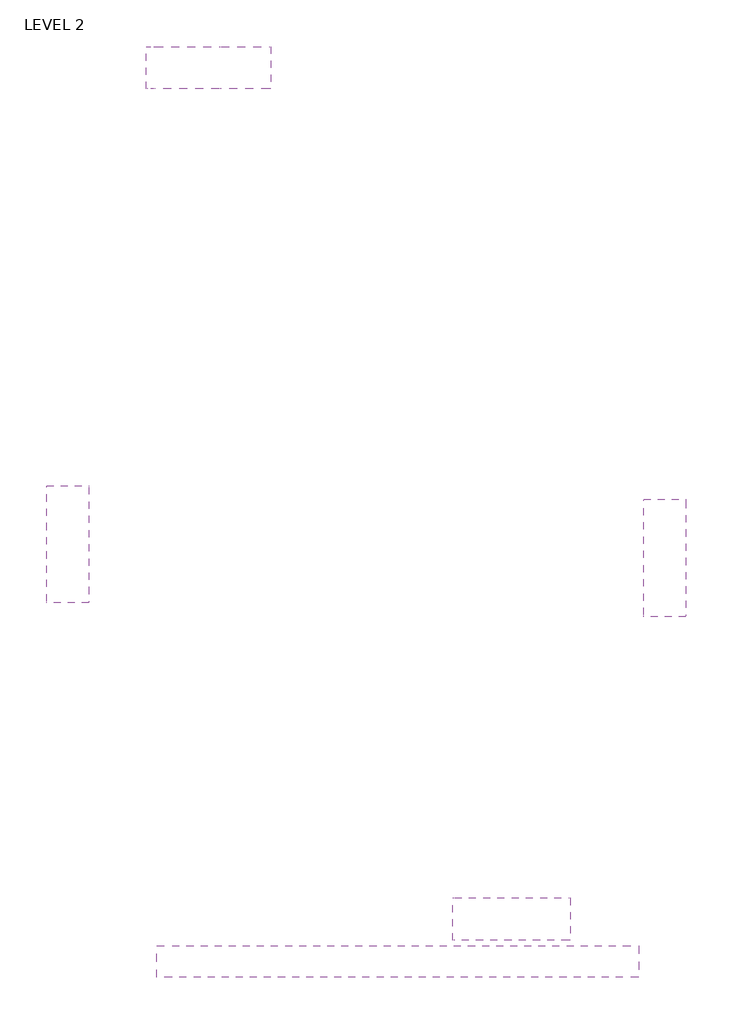
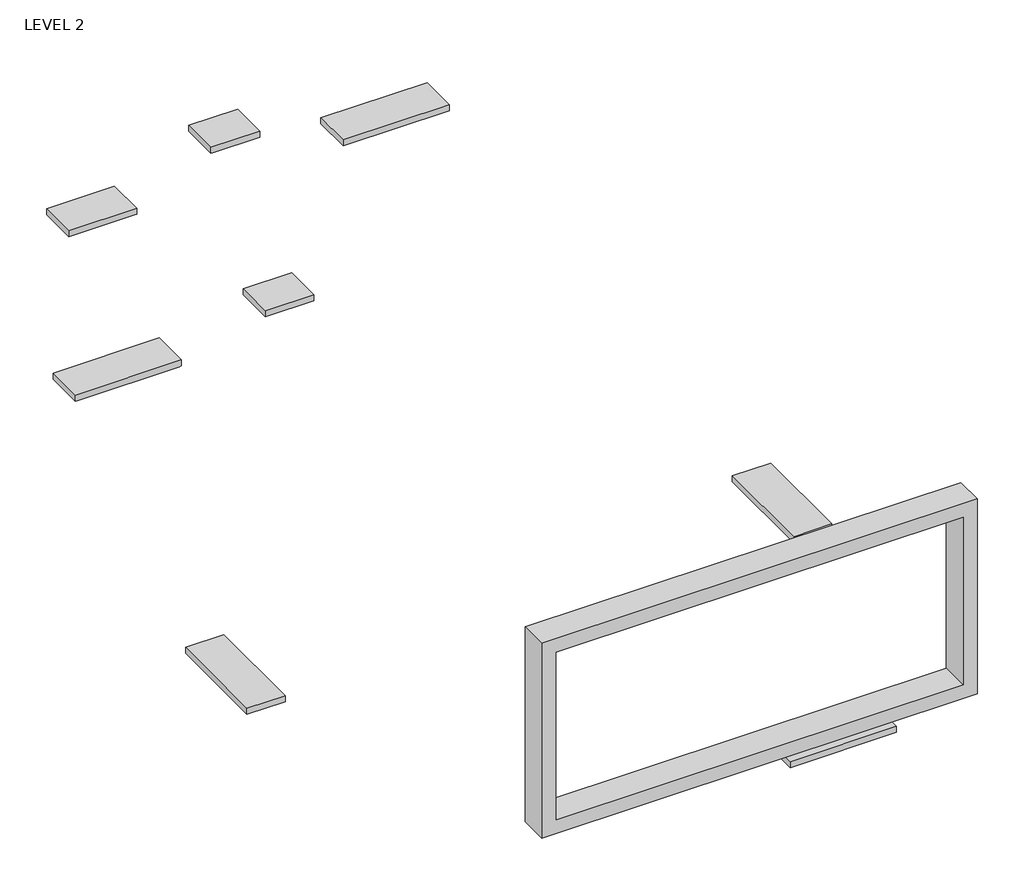
# One storey: 5 proxies.
"""IFC4 building model written with IfcOpenShell, lengths in millimetres."""

from ifc_helpers import new_model, si_unit, origin, place, context, project, spatial, transform, mapped, element, save
from components import generic_models_10_generic_models_10_c1604470, generic_models_5_generic_models_5_57bc8fc0, generic_models_7_generic_models_7_8ab6631d, generic_models_8_generic_models_8_8680fe62, generic_models_9_generic_models_9_de2daabc

model = new_model("IFC4")

# Units and contexts
model_context = context("Model", 3, world=origin())
ifc_project = project(units=[si_unit("LENGTHUNIT", "METRE", prefix="MILLI")], contexts=[model_context])

# Site, building, storey
site = spatial("IfcSite", under=ifc_project)
building = spatial("IfcBuilding", under=site)
storey = spatial("IfcBuildingStorey", under=building, Name="LEVEL 2", Elevation=914.4)

# Proxies
placement = place(None, origin())
generic_models_10_generic_models_10_shape = generic_models_10_generic_models_10_c1604470(model_context)
element("IfcBuildingElementProxy", 1, Name="Generic Models 10 : Generic Models 10", ObjectType="Generic Models 10 : Generic Models 10", at=placement, inside=storey, context=model_context, shape_type="MappedRepresentation", body=[
    mapped(generic_models_10_generic_models_10_shape, transform((0.0, 0.0, 0.0), x_axis=(1.0, 0.0, 0.0), y_axis=(0.0, 1.0, 0.0), z_axis=(0.0, 0.0, 1.0))),
])
generic_models_5_generic_models_5_shape = generic_models_5_generic_models_5_57bc8fc0(model_context)
element("IfcBuildingElementProxy", 2, Name="Generic Models 5 : Generic Models 5", ObjectType="Generic Models 5 : Generic Models 5", at=placement, inside=storey, context=model_context, shape_type="MappedRepresentation", body=[
    mapped(generic_models_5_generic_models_5_shape, transform((0.0, 0.0, 0.0), x_axis=(1.0, 0.0, 0.0), y_axis=(0.0, 1.0, 0.0), z_axis=(0.0, 0.0, 1.0))),
])
generic_models_7_generic_models_7_shape = generic_models_7_generic_models_7_8ab6631d(model_context)
element("IfcBuildingElementProxy", 3, Name="Generic Models 7 : Generic Models 7", ObjectType="Generic Models 7 : Generic Models 7", at=placement, inside=storey, context=model_context, shape_type="MappedRepresentation", body=[
    mapped(generic_models_7_generic_models_7_shape, transform((0.0, 0.0, 0.0), x_axis=(1.0, 0.0, 0.0), y_axis=(0.0, 1.0, 0.0), z_axis=(0.0, 0.0, 1.0))),
])
generic_models_8_generic_models_8_shape = generic_models_8_generic_models_8_8680fe62(model_context)
element("IfcBuildingElementProxy", 4, Name="Generic Models 8 : Generic Models 8", ObjectType="Generic Models 8 : Generic Models 8", at=placement, inside=storey, context=model_context, shape_type="MappedRepresentation", body=[
    mapped(generic_models_8_generic_models_8_shape, transform((0.0, 0.0, 0.0), x_axis=(1.0, 0.0, 0.0), y_axis=(0.0, 1.0, 0.0), z_axis=(0.0, 0.0, 1.0))),
])
generic_models_9_generic_models_9_shape = generic_models_9_generic_models_9_de2daabc(model_context)
element("IfcBuildingElementProxy", 5, Name="Generic Models 9 : Generic Models 9", ObjectType="Generic Models 9 : Generic Models 9", at=placement, inside=storey, context=model_context, shape_type="MappedRepresentation", body=[
    mapped(generic_models_9_generic_models_9_shape, transform((0.0, 0.0, 0.0), x_axis=(1.0, 0.0, 0.0), y_axis=(0.0, 1.0, 0.0), z_axis=(0.0, 0.0, 1.0))),
])

save(model, "model.ifc")

# Revit data of these elements
# Element 1 (IfcBuildingElementProxy, "Generic Models 10 : Generic Models 10")
#   Phase Created = New Construction
# Element 2 (IfcBuildingElementProxy, "Generic Models 5 : Generic Models 5")
#   Phase Created = New Construction
# Element 3 (IfcBuildingElementProxy, "Generic Models 7 : Generic Models 7")
#   Phase Created = New Construction
# Element 4 (IfcBuildingElementProxy, "Generic Models 8 : Generic Models 8")
#   Phase Created = New Construction
# Element 5 (IfcBuildingElementProxy, "Generic Models 9 : Generic Models 9")
#   Phase Created = New Construction
